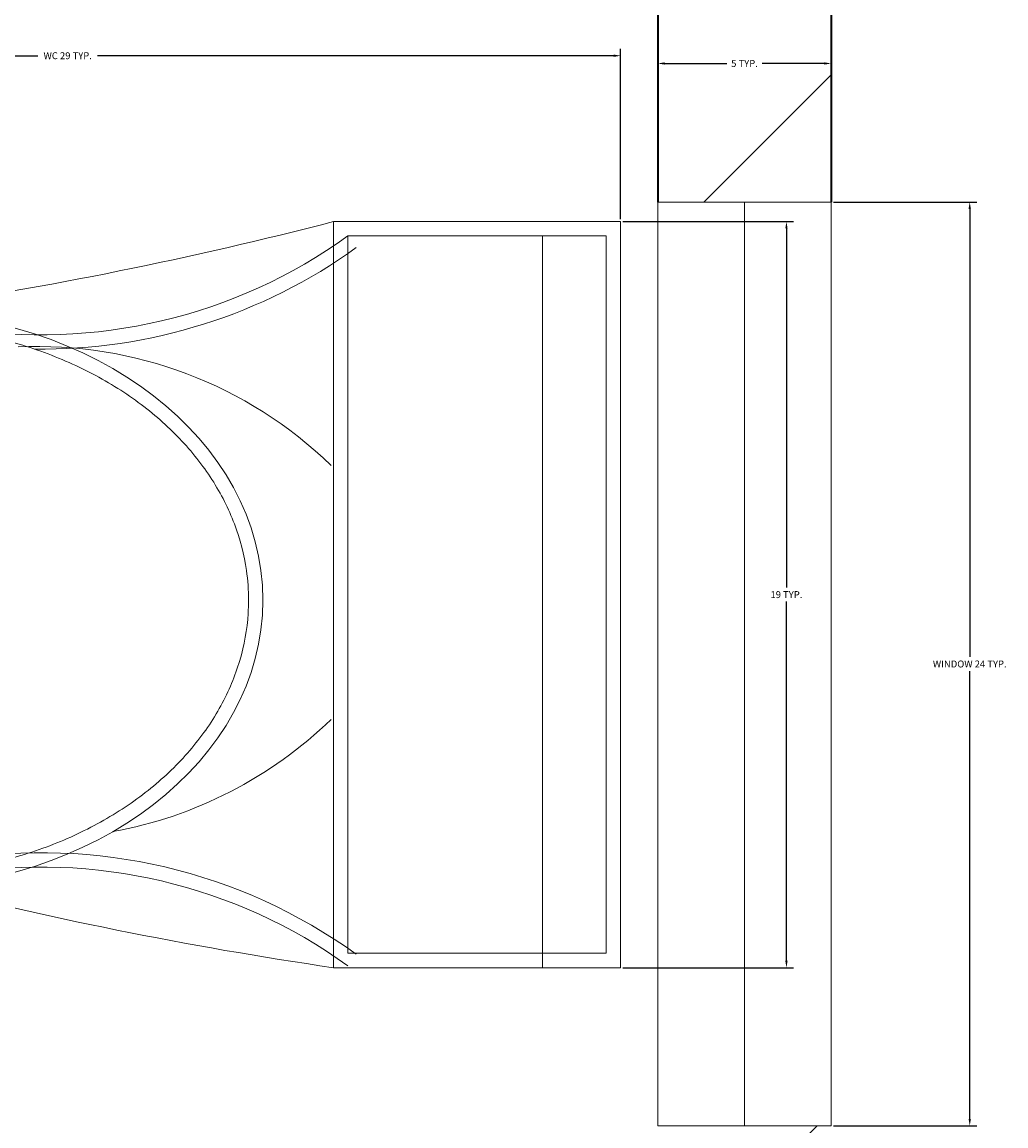
# Model space of a CAD drawing. Units: inches. Extents: x 2168 to 3056, y 1130 to 2629.
# Tile 37 of 42: x 2843 to 2869, y 2217 to 2246. Entities that reach past the tile are written whole.
import ezdxf

# ---------------------------------------------------------------- set-up
doc = ezdxf.new("R2010")
doc.units = ezdxf.units.IN
for name, color, linetype, lineweight in [('A-ANNO-DIMS', 2, 'Continuous', 18), ('A-FLOR-FIXT', 9, 'Continuous', 18), ('A-GLAZ', 201, 'Continuous', 18), ('A-WALL', 7, 'Continuous', 35)]:
    doc.layers.add(name, color=color, linetype=linetype, lineweight=lineweight)
doc.layers.add('A-WALL-PATT', color=143, linetype='Continuous', lineweight=13, true_color=0x7aafdf)
doc.styles.get("Standard").update_dxf_attribs({"font": 'arial.ttf'})
doc.dimstyles.get("Standard").update_dxf_attribs({"dimtxt": 0.18, "dimasz": 0.18, "dimexe": 0.18, "dimexo": 0.0625, "dimgap": 0.09, "dimtad": 0, "dimtih": 1, "dimtoh": 1, "dimdec": 4, "dimzin": 0, "dimdsep": 46, "dimtxsty": 'Standard', "dimcen": 0.09, "dimadec": 0, "dimazin": 0, "dimtfac": 1, "dimtdec": 4, "dimtofl": 0, "dimtmove": 0, "dimatfit": 3, "dimfxl": 1, "dimtolj": 1, "dimtzin": 0, "dimarcsym": 0})

# ---------------------------------------------------------------- blocks, each defined once
blk = doc.blocks.new('A$C31115884')
for p, q in [((0, 200), (0, 0)), ((520, 200), (0, 200)), ((520, 0), (520, 200)), ((10, 190), (10, 10)), ((510, 190), (10, 190)), ((510, 10), (510, 190)), ((510, 54.46), (0, 54.46)), ((10, 10), (510, 10)), ((0, 0), (520, 0))]:
    blk.add_line(p, q)
for centre, radius, start, end in [((2777.7, -204.57), 2807.01, 165.4549, 171.71327), ((3237.04, 904.96), 2807.01, 188.28673, 194.5451), ((-294.54, 403.26), 364.66, 324.20913, 9.34987), ((-294.54, 403.26), 374.66, 324.20913, 9.34987), ((805.79, 403.26), 364.66, 170.65013, 215.79087), ((139.48, 406.23), 293.48, 315.84364, 2.65635), ((805.79, 403.26), 374.66, 179.20365, 215.79087), ((383.57, 406.23), 293.48, 190.27735, 224.15636)]:
    blk.add_arc(centre, radius, start, end)
blk.add_ellipse((256.16, 509.9), major_axis=(0, -260.67), ratio=0.772727)
blk.add_open_spline([(256.16, 259.23), (263.08, 259.23), (269.99, 259.72), (287.81, 262.27), (298.65, 265.08), (319.86, 273.12), (330.22, 278.35), (350.15, 291.13), (359.72, 298.67), (377.75, 315.86), (386.21, 325.51), (401.75, 346.63), (408.82, 358.1), (421.35, 382.52), (426.79, 395.46), (435.87, 422.42), (439.5, 436.43), (444.83, 465.08), (446.52, 479.72), (447.92, 509.17), (447.62, 523.97), (445.03, 553.27), (442.74, 567.77), (436.26, 596.01), (432.07, 609.74), (421.91, 636.02), (415.95, 648.56), (402.47, 672.06), (394.95, 683.02), (378.6, 703.01), (369.78, 712.05), (351.11, 727.96), (341.27, 734.82), (320.89, 746.2), (310.35, 750.71), (288.88, 757.29), (277.96, 759.35), (256, 760.98), (244.98, 760.56), (223.13, 757.22), (212.3, 754.31), (191.14, 746.06), (180.8, 740.72), (160.94, 727.75), (151.41, 720.12), (133.48, 702.75), (125.07, 693.02), (109.65, 671.74), (102.63, 660.2), (90.25, 635.66), (84.88, 622.67), (75.95, 595.62), (72.4, 581.57), (67.24, 552.87), (65.63, 538.21), (64.4, 508.76), (64.79, 493.96), (67.54, 464.68), (69.91, 450.2), (76.56, 422.03), (80.83, 408.34), (91.13, 382.16), (97.16, 369.68), (110.77, 346.32), (118.35, 335.44), (134.81, 315.6), (143.69, 306.65), (162.44, 290.93), (172.32, 284.16), (192.75, 272.98), (203.31, 268.57), (224.81, 262.2), (235.75, 260.25), (249.87, 259.33), (253.02, 259.23), (256.16, 259.23)], degree=3, knots=[0, 0, 0, 0, 0.110105, 0.110105, 0.285049, 0.285049, 0.459994, 0.459994, 0.634938, 0.634938, 0.809882, 0.809882, 0.984827, 0.984827, 1.159771, 1.159771, 1.334715, 1.334715, 1.50966, 1.50966, 1.684604, 1.684604, 1.859549, 1.859549, 2.034493, 2.034493, 2.209437, 2.209437, 2.384382, 2.384382, 2.559326, 2.559326, 2.73427, 2.73427, 2.909215, 2.909215, 3.084159, 3.084159, 3.259103, 3.259103, 3.434048, 3.434048, 3.608992, 3.608992, 3.783936, 3.783936, 3.958881, 3.958881, 4.133825, 4.133825, 4.30877, 4.30877, 4.483714, 4.483714, 4.658658, 4.658658, 4.833603, 4.833603, 5.008547, 5.008547, 5.183491, 5.183491, 5.358436, 5.358436, 5.53338, 5.53338, 5.708324, 5.708324, 5.883269, 5.883269, 6.058213, 6.058213, 6.233158, 6.233158, 6.283185, 6.283185, 6.283185, 6.283185])
blk = doc.blocks.new('WIN-24')
for p, q in [((0, 0), (0, 4.5)), ((0, 4.5), (0, 2.25)), ((0, 4.5), (24, 4.5)), ((24, 2.25), (24, 4.5)), ((24, 4.5), (24, 0)), ((0, 2.25), (24, 2.25)), ((24, 0), (0, 0))]:
    blk.add_line(p, q)
blk = doc.blocks.new('*D20')
at = {"layer": 'A-ANNO-DIMS', "color": 0, "lineweight": -2, "transparency": 16777216}
for p, q in [((2830.107, 2240.907), (2830.107, 2245.333)), ((2858.827, 2240.907), (2858.827, 2245.333)), ((2830.287, 2245.153), (2843.691, 2245.153)), ((2858.647, 2245.153), (2845.243, 2245.153))]:
    blk.add_line(p, q, dxfattribs=at)
at = {"layer": 'A-ANNO-DIMS', "color": 0, "transparency": 16777216}
for points in [[(2830.287, 2245.183), (2830.287, 2245.123), (2830.107, 2245.153)], [(2858.647, 2245.183), (2858.647, 2245.123), (2858.827, 2245.153)]]:
    blk.add_solid(points, dxfattribs=at)
at = {"layer": 'Defpoints', "color": 0, "transparency": 16777216}
for p in [(2830.107, 2245.153), (2830.107, 2240.845), (2858.827, 2240.845)]:
    blk.add_point(p, dxfattribs=at)
at = {"layer": 'A-ANNO-DIMS', "color": 0, "transparency": 16777216, "insert": (2844.467, 2245.153), "char_height": 0.18, "attachment_point": 5}
blk.add_mtext('\\A1;WC 29 TYP.', dxfattribs=at)
blk = doc.blocks.new('*D21')
at = {"layer": 'A-ANNO-DIMS', "color": 0, "lineweight": -2, "transparency": 16777216}
for p, q in [((2858.89, 2240.845), (2863.315, 2240.845)), ((2863.135, 2240.665), (2863.135, 2231.336)), ((2863.135, 2221.643), (2863.135, 2230.972)), ((2858.89, 2221.463), (2863.315, 2221.463))]:
    blk.add_line(p, q, dxfattribs=at)
at = {"layer": 'A-ANNO-DIMS', "color": 0, "transparency": 16777216}
for points in [[(2863.105, 2240.665), (2863.165, 2240.665), (2863.135, 2240.845)], [(2863.105, 2221.643), (2863.165, 2221.643), (2863.135, 2221.463)]]:
    blk.add_solid(points, dxfattribs=at)
at = {"layer": 'Defpoints', "color": 0, "transparency": 16777216}
for p in [(2858.827, 2240.845), (2863.135, 2240.845), (2858.827, 2221.463)]:
    blk.add_point(p, dxfattribs=at)
at = {"layer": 'A-ANNO-DIMS', "color": 0, "transparency": 16777216, "insert": (2863.135, 2231.154), "char_height": 0.18, "attachment_point": 5}
blk.add_mtext('\\A1;19 TYP.', dxfattribs=at)
blk = doc.blocks.new('*D32')
at = {"layer": 'A-ANNO-DIMS', "color": 0, "lineweight": -2, "transparency": 16777216}
for p, q in [((2864.358, 2241.352), (2868.076, 2241.352)), ((2867.896, 2241.172), (2867.896, 2229.535)), ((2867.896, 2217.532), (2867.896, 2229.169)), ((2864.358, 2217.352), (2868.076, 2217.352))]:
    blk.add_line(p, q, dxfattribs=at)
at = {"layer": 'A-ANNO-DIMS', "color": 0, "transparency": 16777216}
for points in [[(2867.866, 2241.172), (2867.926, 2241.172), (2867.896, 2241.352)], [(2867.866, 2217.532), (2867.926, 2217.532), (2867.896, 2217.352)]]:
    blk.add_solid(points, dxfattribs=at)
at = {"layer": 'Defpoints', "color": 0, "transparency": 16777216}
for p in [(2864.296, 2241.352), (2864.296, 2217.352), (2867.896, 2217.352)]:
    blk.add_point(p, dxfattribs=at)
at = {"layer": 'A-ANNO-DIMS', "color": 0, "transparency": 16777216, "insert": (2867.896, 2229.352), "char_height": 0.18, "attachment_point": 5}
blk.add_mtext('\\A1;WINDOW 24 TYP.', dxfattribs=at)
blk = doc.blocks.new('*D33')
at = {"layer": 'A-ANNO-DIMS', "color": 0, "lineweight": -2, "transparency": 16777216}
for p, q in [((2859.796, 2241.414), (2859.796, 2245.132)), ((2864.296, 2241.414), (2864.296, 2245.132)), ((2859.976, 2244.952), (2861.588, 2244.952)), ((2864.116, 2244.952), (2862.504, 2244.952))]:
    blk.add_line(p, q, dxfattribs=at)
at = {"layer": 'A-ANNO-DIMS', "color": 0, "transparency": 16777216}
for points in [[(2859.976, 2244.982), (2859.976, 2244.922), (2859.796, 2244.952)], [(2864.116, 2244.982), (2864.116, 2244.922), (2864.296, 2244.952)]]:
    blk.add_solid(points, dxfattribs=at)
at = {"layer": 'Defpoints', "color": 0, "transparency": 16777216}
for p in [(2864.296, 2244.952), (2859.796, 2241.352), (2864.296, 2241.352)]:
    blk.add_point(p, dxfattribs=at)
at = {"layer": 'A-ANNO-DIMS', "color": 0, "transparency": 16777216, "insert": (2862.046, 2244.952), "char_height": 0.18, "attachment_point": 5}
blk.add_mtext('\\A1;5 TYP.', dxfattribs=at)

msp = doc.modelspace()

# ---------------------------------------------------------------- hatches: boundary and pattern name
at = {"layer": 'A-WALL-PATT'}
h = msp.add_hatch(dxfattribs=at)
h.set_pattern_fill('ANSI32', color=256)
h.paths.add_polyline_path([(2463.796, 2409.389), (2467.387, 2409.389), (2467.387, 2413.889), (2454.768, 2413.889), (2454.768, 2411.639), (2454.768, 2409.389), (2459.296, 2409.389), (2459.296, 2265.389), (2455.644, 2265.389), (2455.644, 2260.889), (2467.349, 2260.889), (2467.349, 2263.139), (2467.349, 2265.389), (2463.796, 2265.389)])
h.paths.add_polyline_path([(2431.596, 2413.889), (2409.647, 2413.889), (2409.647, 2409.389), (2431.596, 2409.389), (2431.596, 2411.639)])
h.paths.add_polyline_path([(2349.647, 2413.889), (2331.796, 2413.889), (2331.796, 2362.671), (2336.296, 2362.671), (2336.296, 2409.389), (2349.647, 2409.389), (2349.647, 2411.639)])
h.paths.add_polyline_path([(2634.149, 2411.639), (2634.149, 2413.889), (2562.293, 2413.889), (2562.293, 2409.389), (2595.796, 2409.389), (2595.796, 2280.309), (2595.826, 2280.309), (2595.826, 2265.389), (2499.91, 2265.389), (2499.91, 2260.889), (2550.796, 2260.889), (2550.796, 2117.308), (2555.296, 2117.308), (2555.296, 2168.08), (2571.93, 2168.08), (2571.93, 2176.889), (2559.796, 2176.889), (2559.796, 2256.389), (2640.796, 2256.389), (2640.796, 2176.889), (2626.428, 2176.889), (2626.428, 2168.08), (2645.296, 2168.08), (2645.296, 2116.637), (2649.796, 2116.637), (2649.796, 2260.889), (2691.251, 2260.889), (2691.251, 2263.139), (2691.251, 2265.389), (2670.655, 2265.389), (2670.655, 2265.365), (2600.296, 2265.365), (2600.296, 2280.258), (2600.296, 2409.389), (2634.149, 2409.389)])
h.paths.add_polyline_path([(2600.296, 2473.889), (2612.84, 2473.889), (2612.84, 2478.389), (2572.636, 2478.389), (2572.636, 2473.889), (2595.796, 2473.889), (2595.796, 2413.889), (2600.296, 2413.889)])
h.paths.add_polyline_path([(2535.796, 2473.889), (2548.636, 2473.889), (2548.636, 2478.389), (2531.396, 2478.389), (2531.396, 2413.889), (2521.6, 2413.889), (2521.6, 2409.389), (2539.239, 2409.389), (2539.239, 2411.639), (2539.239, 2413.889), (2535.796, 2413.889)])
h.paths.add_polyline_path([(2664.796, 2478.389), (2636.84, 2478.389), (2636.84, 2473.889), (2660.296, 2473.889), (2660.296, 2413.889), (2656.165, 2413.889), (2656.165, 2409.389), (2671.684, 2409.389), (2671.684, 2411.639), (2671.684, 2413.889), (2664.796, 2413.889)])
h.paths.add_polyline_path([(2705.942, 2413.889), (2695.684, 2413.889), (2695.684, 2409.389), (2705.942, 2409.389)])
h.paths.add_polyline_path([(2741.35, 2413.889), (2728.733, 2413.889), (2728.733, 2411.639), (2728.733, 2409.389), (2732.296, 2409.389), (2732.296, 2265.389), (2725.733, 2265.389), (2725.733, 2260.889), (2740.917, 2260.889), (2740.917, 2263.139), (2740.917, 2265.389), (2736.796, 2265.389), (2736.796, 2409.389), (2741.35, 2409.389)])
h.paths.add_polyline_path([(2785.655, 2413.889), (2764.546, 2413.889), (2764.486, 2409.389), (2785.655, 2409.389), (2785.655, 2411.639)])
h.paths.add_polyline_path([(2864.296, 2413.889), (2845.655, 2413.889), (2845.655, 2409.389), (2859.796, 2409.389), (2859.796, 2368.425), (2864.296, 2368.425)])
h.paths.add_polyline_path([(2864.296, 2308.425), (2862.046, 2308.425), (2859.796, 2308.425), (2859.796, 2265.389), (2774.483, 2265.389), (2774.483, 2263.139), (2774.483, 2260.889), (2781.796, 2260.889), (2781.796, 2226.654), (2786.296, 2226.654), (2786.296, 2260.889), (2859.796, 2260.889), (2859.796, 2241.352), (2864.296, 2241.352)])
h.paths.add_polyline_path([(2864.296, 2217.352), (2862.046, 2217.352), (2859.796, 2217.352), (2859.796, 2200.889), (2786.296, 2200.889), (2786.296, 2205.931), (2784.046, 2205.931), (2781.796, 2205.931), (2781.796, 2150.974), (2786.296, 2150.974), (2786.296, 2161.889), (2859.796, 2161.889), (2859.796, 2144.419), (2864.296, 2144.419)])
h.paths.add_polyline_path([(2859.796, 2196.389), (2859.796, 2166.389), (2786.296, 2166.389), (2786.296, 2196.389)], flags=16)
h.paths.add_polyline_path([(2864.296, 2108.419), (2862.046, 2108.419), (2859.796, 2108.419), (2859.796, 2080.889), (2786.296, 2080.889), (2786.296, 2111.993), (2781.796, 2111.993), (2781.796, 2080.889), (2649.796, 2080.889), (2649.796, 2086.036), (2647.546, 2086.036), (2645.296, 2086.036), (2645.296, 2071.739), (2649.796, 2071.739), (2649.796, 2076.389), (2781.796, 2076.389), (2781.796, 2041.792), (2786.296, 2041.792), (2786.296, 2076.389), (2859.796, 2076.389), (2859.796, 2058.577), (2864.296, 2058.577)])
h.paths.add_polyline_path([(2864.296, 2022.577), (2859.796, 2022.577), (2859.796, 1992.389), (2786.296, 1992.389), (2786.296, 1999.573), (2781.796, 1999.573), (2781.796, 1848.085), (2784.046, 1848.085), (2786.296, 1848.085), (2786.296, 1851.389), (2859.796, 1851.389), (2859.796, 1838.258), (2864.296, 1838.258)], flags=17)
h.paths.add_polyline_path([(2859.796, 1987.889), (2859.796, 1855.889), (2786.296, 1855.889), (2786.296, 1987.889)], flags=16)
h.paths.add_polyline_path([(2823.046, 1987.889), (2841.421, 1921.889), (2823.046, 1855.889)], flags=0)
h.paths.add_polyline_path([(2864.296, 1814.258), (2859.796, 1814.258), (2859.796, 1791.389), (2786.296, 1791.389), (2786.296, 1825.658), (2784.046, 1825.658), (2781.796, 1825.658), (2781.796, 1791.389), (2720.155, 1791.389), (2720.155, 1791.265), (2649.796, 1791.265), (2649.796, 1806.159), (2649.796, 2038.983), (2647.546, 2038.983), (2645.296, 2038.983), (2645.296, 1783.925), (2649.796, 1783.925), (2649.796, 1786.889), (2781.796, 1786.889), (2781.796, 1746.789), (2786.296, 1746.789), (2786.296, 1786.889), (2859.796, 1786.889), (2859.796, 1770.083), (2864.296, 1770.083)])
h.paths.add_polyline_path([(2864.296, 1734.083), (2862.046, 1734.083), (2859.796, 1734.083), (2859.796, 1705.889), (2786.296, 1705.889), (2786.296, 1714.166), (2781.796, 1714.166), (2781.796, 1660.527), (2786.296, 1660.527), (2786.296, 1666.889), (2859.796, 1666.889), (2859.796, 1648.342), (2864.296, 1648.342)])
h.paths.add_polyline_path([(2786.296, 1701.389), (2859.796, 1701.389), (2859.796, 1671.389), (2786.296, 1671.389)], flags=16)
h.paths.add_polyline_path([(2649.796, 1756.576), (2647.546, 1756.576), (2645.296, 1756.576), (2645.296, 1606.889), (2555.296, 1606.889), (2555.296, 1749.513), (2553.046, 1749.513), (2550.796, 1749.513), (2550.796, 1606.889), (2503.006, 1606.889), (2503.006, 1604.639), (2503.006, 1602.389), (2595.796, 1602.389), (2595.849, 1602.389), (2595.849, 1587.495), (2595.796, 1458.389), (2561.502, 1458.389), (2561.502, 1456.139), (2561.502, 1453.889), (2595.796, 1453.889), (2595.796, 1381.889), (2573.438, 1381.889), (2573.438, 1377.389), (2613.01, 1377.389), (2613.01, 1379.639), (2613.01, 1381.889), (2600.296, 1381.889), (2600.296, 1453.889), (2634.327, 1453.889), (2634.327, 1458.389), (2600.296, 1458.389), (2600.296, 1602.389), (2670.655, 1602.389), (2694.095, 1602.389), (2694.095, 1606.889), (2649.796, 1606.889)])
h.paths.add_polyline_path([(2736.796, 1602.389), (2741.562, 1602.389), (2741.562, 1606.889), (2726.203, 1606.889), (2726.203, 1604.639), (2726.203, 1602.389), (2732.296, 1602.389), (2732.296, 1458.389), (2727.899, 1458.389), (2727.899, 1453.889), (2740.821, 1453.889), (2740.821, 1456.139), (2740.821, 1458.389), (2736.796, 1458.389)])
h.paths.add_polyline_path([(2859.796, 1606.889), (2786.296, 1606.889), (2786.296, 1637.334), (2784.046, 1637.334), (2781.796, 1637.334), (2781.796, 1606.889), (2775.612, 1606.889), (2775.612, 1602.389), (2859.796, 1602.389)])
h.paths.add_polyline_path([(2864.296, 1624.342), (2862.046, 1624.342), (2859.796, 1624.342), (2859.796, 1570.39), (2864.296, 1570.39)])
h.paths.add_polyline_path([(2864.296, 1510.39), (2862.046, 1510.39), (2859.796, 1510.39), (2859.796, 1458.389), (2846.735, 1458.389), (2846.735, 1456.139), (2846.735, 1453.889), (2864.296, 1453.889)])
h.paths.add_polyline_path([(2786.735, 1458.389), (2765.444, 1458.389), (2765.444, 1453.889), (2786.735, 1453.889)])
h.paths.add_polyline_path([(2706.004, 1458.389), (2695.36, 1458.389), (2695.36, 1453.889), (2706.004, 1453.889), (2706.004, 1456.139)])
h.paths.add_polyline_path([(2671.36, 1456.139), (2671.36, 1458.389), (2655.986, 1458.389), (2655.986, 1456.139), (2655.986, 1453.889), (2660.296, 1453.889), (2660.296, 1381.889), (2637.01, 1381.889), (2637.01, 1377.389), (2664.796, 1377.389), (2664.796, 1453.889), (2671.36, 1453.889)], flags=17)
h.paths.add_polyline_path([(2539.829, 1458.389), (2520.237, 1458.389), (2520.237, 1453.889), (2531.296, 1453.889), (2531.296, 1377.389), (2546.449, 1377.389), (2546.449, 1379.639), (2546.449, 1381.889), (2535.796, 1381.889), (2535.796, 1453.889), (2539.829, 1453.889)], flags=17)
h.paths.add_polyline_path([(2496.237, 1458.389), (2489.13, 1458.389), (2489.13, 1453.889), (2496.237, 1453.889), (2496.237, 1456.139)])
h.paths.add_polyline_path([(2467.433, 1456.139), (2467.433, 1458.389), (2463.796, 1458.389), (2463.796, 1602.389), (2468.242, 1602.389), (2468.242, 1605.7), (2468.242, 1606.889), (2454.602, 1606.889), (2454.602, 1602.389), (2459.296, 1602.389), (2459.296, 1458.389), (2454.24, 1458.389), (2454.24, 1453.889), (2467.433, 1453.889)])
h.paths.add_polyline_path([(2431.601, 1456.139), (2431.601, 1458.389), (2411.386, 1458.389), (2411.386, 1453.889), (2431.601, 1453.889)])
h.paths.add_polyline_path([(2351.386, 1458.389), (2336.296, 1458.389), (2336.296, 1490.693), (2334.046, 1490.693), (2331.796, 1490.693), (2331.796, 1453.889), (2351.386, 1453.889), (2351.386, 1456.139)])
h.paths.add_polyline_path([(2336.296, 1629.705), (2331.796, 1629.705), (2331.796, 1552.317), (2336.296, 1552.317), (2336.296, 1602.389), (2406.655, 1602.389), (2423.472, 1602.389), (2423.472, 1606.889), (2418.796, 1606.889), (2418.796, 1643.678), (2416.546, 1643.678), (2414.296, 1643.678), (2414.296, 1606.889), (2336.296, 1606.889)])
h.paths.add_polyline_path([(2418.796, 1714.384), (2414.296, 1714.384), (2414.296, 1705.889), (2336.296, 1705.889), (2336.296, 1731.324), (2334.046, 1731.324), (2331.796, 1731.324), (2331.796, 1653.705), (2334.046, 1653.705), (2336.296, 1653.705), (2336.296, 1666.889), (2414.296, 1666.889), (2414.296, 1663.589), (2418.796, 1663.589)])
h.paths.add_polyline_path([(2336.296, 1701.389), (2414.296, 1701.389), (2414.296, 1671.389), (2336.296, 1671.389)], flags=16)
h.paths.add_polyline_path([(2555.296, 2040.059), (2550.796, 2040.059), (2550.796, 1791.389), (2550.561, 1791.205), (2480.202, 1791.205), (2418.796, 1791.389), (2418.796, 1825.448), (2416.546, 1825.448), (2414.296, 1825.448), (2414.296, 1791.389), (2336.296, 1791.389), (2336.296, 1806.409), (2331.796, 1806.409), (2331.796, 1767.324), (2336.296, 1767.324), (2336.296, 1786.889), (2414.296, 1786.889), (2414.296, 1745.457), (2418.796, 1745.457), (2418.796, 1786.889), (2550.796, 1786.889), (2550.796, 1783.011), (2555.296, 1783.011)])
h.paths.add_polyline_path([(2418.796, 1923.389), (2423.207, 1923.389), (2423.207, 1925.639), (2423.207, 1927.889), (2418.796, 1927.889), (2418.796, 2000.048), (2414.296, 2000.048), (2414.296, 1992.389), (2336.296, 1992.389), (2336.296, 1987.889), (2414.296, 1987.889), (2414.296, 1855.889), (2336.296, 1855.889), (2336.296, 1851.389), (2414.296, 1851.389), (2414.296, 1846.759), (2418.796, 1846.759)], flags=17)
h.paths.add_polyline_path([(2336.296, 2019.294), (2334.046, 2019.294), (2331.796, 2019.294), (2331.796, 1830.409), (2336.296, 1830.409)], flags=17)
h.paths.add_polyline_path([(2550.796, 1927.889), (2453.541, 1927.889), (2453.541, 1925.639), (2453.541, 1923.389), (2550.796, 1923.389)], flags=17)
h.paths.add_polyline_path([(2744.987, 1927.889), (2649.796, 1927.889), (2649.796, 1923.389), (2744.987, 1923.389), (2744.987, 1925.639)], flags=17)
h.paths.add_polyline_path([(2555.296, 2086.458), (2553.046, 2086.458), (2550.796, 2086.458), (2550.796, 2080.889), (2418.796, 2080.889), (2336.296, 2080.889), (2336.296, 2115.399), (2334.046, 2115.399), (2331.796, 2115.399), (2331.796, 2055.294), (2336.296, 2055.294), (2336.296, 2076.389), (2550.796, 2076.389), (2550.796, 2071.538), (2555.296, 2071.538)])
h.paths.add_polyline_path([(2418.796, 2121.389), (2414.296, 2121.389), (2414.296, 2080.889), (2418.796, 2080.889)])
h.paths.add_polyline_path([(2418.796, 2076.389), (2414.296, 2076.389), (2414.296, 2035.123), (2418.796, 2035.123)])
h.paths.add_polyline_path([(2422.868, 2263.139), (2422.868, 2265.389), (2406.655, 2265.389), (2406.655, 2265.359), (2336.296, 2265.359), (2336.296, 2280.252), (2336.296, 2302.671), (2334.046, 2302.671), (2331.796, 2302.671), (2331.796, 2246.853), (2336.296, 2246.853), (2336.296, 2260.889), (2414.296, 2260.889), (2414.296, 2223.996), (2418.796, 2223.996), (2418.796, 2260.889), (2422.868, 2260.889)])
h.paths.add_polyline_path([(2418.796, 2204.783), (2416.546, 2204.783), (2414.296, 2204.783), (2414.296, 2200.889), (2336.296, 2200.889), (2336.296, 2220.853), (2331.796, 2220.853), (2331.796, 2151.399), (2336.296, 2151.399), (2336.296, 2161.889), (2414.296, 2161.889), (2414.296, 2153.726), (2418.796, 2153.726)])
h.paths.add_polyline_path([(2414.296, 2196.389), (2414.296, 2166.389), (2336.296, 2166.389), (2336.296, 2196.389)], flags=16)
h.paths.add_polyline_path([(2375.296, 2181.389), (2336.296, 2166.389), (2336.296, 2196.389)], flags=0)
h.paths.add_polyline_path([(2809.595, 2172.34), (2838.804, 2172.34), (2838.804, 2190.997), (2809.595, 2190.997)], flags=8)
h.paths.add_polyline_path([(2849.75, 1919.585), (2849.75, 1952.672), (2831.093, 1952.672), (2831.093, 1919.585)], flags=8)
h.paths.add_polyline_path([(2808.875, 1901.967), (2808.875, 1937.85), (2790.149, 1937.85), (2790.149, 1901.967)], flags=8)
h.paths.add_polyline_path([(2806.285, 1671.896), (2835.493, 1671.896), (2835.493, 1690.553), (2806.285, 1690.553)], flags=8)
h.paths.add_polyline_path([(2353.186, 1676.549), (2382.395, 1676.549), (2382.395, 1695.207), (2353.186, 1695.207)], flags=8)
h.paths.add_polyline_path([(2360.083, 1832.308), (2389.241, 1832.308), (2389.241, 1850.966), (2360.083, 1850.966)], flags=25)
h.paths.add_polyline_path([(2354.822, 2167.823), (2384.031, 2167.823), (2384.031, 2186.481), (2354.822, 2186.481)], flags=8)

# ---------------------------------------------------------------- linework, layer by layer
at = {"layer": 'A-WALL'}
for p, q in [((2864.296, 2308.425), (2864.296, 2241.352)), ((2859.796, 2260.889), (2859.796, 2241.352))]:
    msp.add_line(p, q, dxfattribs=at)

# ---------------------------------------------------------------- block references
at = {"layer": 'A-FLOR-FIXT', "xscale": 0.0372717239612423, "yscale": 0.0372717239612423, "zscale": 0.0372717239612423, "rotation": 89.99999999999999}
msp.add_blockref('A$C31115884', (2858.827, 2221.463), dxfattribs=at)
at = {"layer": 'A-GLAZ', "rotation": 270}
msp.add_blockref('WIN-24', (2859.796, 2241.352), dxfattribs=at)

# ---------------------------------------------------------------- dimensions: what is measured, and where the dimension line sits
at = {"layer": 'A-ANNO-DIMS'}
for base, p1, p2, angle, text, picture, middle in [((2830.107, 2245.153), (2858.827, 2240.845), (2830.107, 2240.845), 180, 'WC <> TYP.', '*D20', (2844.467, 2245.153)), ((2867.896, 2217.352), (2864.296, 2241.352), (2864.296, 2217.352), 270, 'WINDOW <> TYP.', '*D32', (2867.896, 2229.352)), ((2863.135, 2240.845), (2858.827, 2221.463), (2858.827, 2240.845), 90, '<> TYP.', '*D21', (2863.135, 2231.154))]:
    dim = msp.add_linear_dim(base=base, p1=p1, p2=p2, angle=angle, text=text, dimstyle='Standard', override={"dimdec": 0, "dimlfac": 1, "dimrnd": 0, "dimzin": 0, "dimdsep": 46, "dimlunit": 2}, dxfattribs=at)
    dim.commit()
    dim.dimension.update_dxf_attribs({"geometry": picture, "text_midpoint": middle})
dim = msp.add_linear_dim(base=(2864.29575579, 2244.951995614), p1=(2859.79575579, 2241.351995614), p2=(2864.29575579, 2241.351995614), text='<> TYP.', dimstyle='Standard', override={"dimdec": 0, "dimlfac": 1, "dimrnd": 0, "dimzin": 0, "dimdsep": 46, "dimlunit": 2}, dxfattribs=at)
dim.commit()
dim.dimension.update_dxf_attribs({"geometry": '*D33', "text_midpoint": (2862.04575579, 2244.951995614)})

doc.saveas('drawing.dxf')
